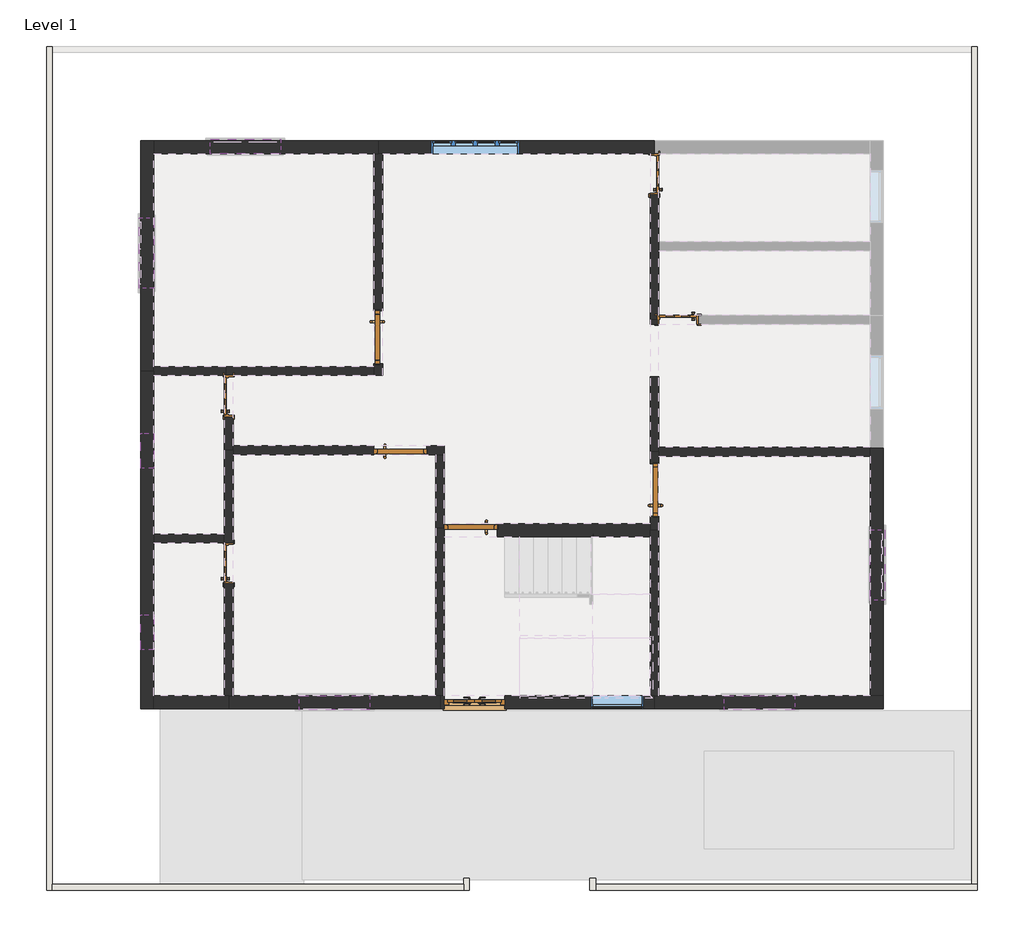
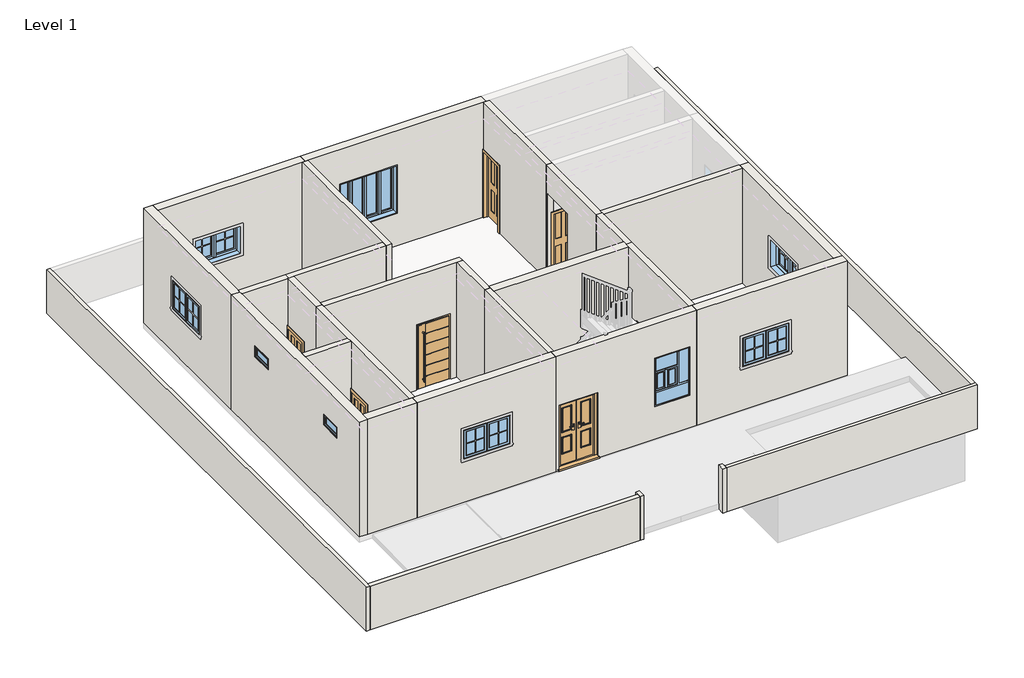
# One storey, part 1 of 2: 30 walls, 9 doors, 9 windows.
"""IFC4 building model written with IfcOpenShell, lengths in millimetres."""

from ifc_helpers import new_model, si_unit, frame, origin, place, context, project, spatial, polyline, outline, extrude, faceted_brep, transform, mapped, element, save
from components import door_3_44036f4b, door_3_3562bf2b, door_a196e7a2, door_f6085f53, door_a03dd1d4, door_7109d6db, m_fixed_2_dd9f9b20, m_window_awning_double_horizontal_4_8afcb0b2, m_window_awning_double_horizontal_4_e2f7b2f6, m_window_casement_double_sash_variable_3_661e274a, m_window_casement_multi_sash_horizontal_5_4f9d37b3

model = new_model("IFC4")

# Units and contexts
model_context = context("Model", 3, world=origin())
ifc_project = project(units=[si_unit("LENGTHUNIT", "METRE", prefix="MILLI")], contexts=[model_context])

# Site, building, storey
site = spatial("IfcSite", under=ifc_project)
building = spatial("IfcBuilding", under=site)
storey = spatial("IfcBuildingStorey", under=building, Name="Level 1", Elevation=0.0)

# Doors
placement = place(None, origin())
door_3_shape = door_3_44036f4b(model_context)
element("IfcDoor", 1, ObjectType="3'", at=placement, inside=storey, context=model_context, shape_type="MappedRepresentation", body=[
    mapped(door_3_shape, transform((-14176.5794909, 1946.4381491, 0.0), x_axis=(0.0, -1.0, 0.0), y_axis=(1.0, 0.0, 0.0), z_axis=(0.0, 0.0, 1.0))),
])
element("IfcDoor", 2, ObjectType="3'", at=placement, inside=storey, context=model_context, shape_type="MappedRepresentation", body=[
    mapped(door_3_shape, transform((-13795.5794909, -9.3618509, 0.0), x_axis=(1.0, 0.0, 0.0), y_axis=(0.0, 1.0, 0.0), z_axis=(0.0, 0.0, 1.0))),
])
element("IfcDoor", 3, ObjectType="3'", at=placement, inside=storey, context=model_context, shape_type="MappedRepresentation", body=[
    mapped(door_3_shape, transform((-9401.3794909, -695.1618509, 0.0), x_axis=(0.0, 1.0, 0.0), y_axis=(-1.0, 0.0, 0.0), z_axis=(0.0, 0.0, 1.0))),
])
door_3_2_shape = door_3_3562bf2b(model_context)
element("IfcDoor", 4, ObjectType="3'", at=placement, inside=storey, context=model_context, shape_type="MappedRepresentation", body=[
    mapped(door_3_2_shape, transform((-12576.3794909, -1393.6618509, 0.0), x_axis=(-1.0, 0.0, 0.0), y_axis=(0.0, -1.0, 0.0), z_axis=(0.0, 0.0, 1.0))),
])
door_shape = door_a196e7a2(model_context)
door_2_shape = door_f6085f53(model_context)
element("IfcDoor", 5, ObjectType="ExtDbl (8) : 3'5\"", at=placement, inside=storey, context=model_context, shape_type="MappedRepresentation", body=[
    mapped(door_shape, transform((-12512.8794909, -4365.4618509, 0.0), x_axis=(-1.0, 0.0, 0.0), y_axis=(0.0, -1.0, 0.0), z_axis=(0.0, 0.0, 1.0))),
    mapped(door_2_shape, transform((-12512.8794909, -4365.4618509, 0.0), x_axis=(-1.0, 0.0, 0.0), y_axis=(0.0, -1.0, 0.0), z_axis=(0.0, 0.0, 1.0))),
])
door_4_shape = door_a03dd1d4(model_context)
element("IfcDoor", 6, ObjectType="M_Door-Interior-Single-4_Panel-Wood : 2'2\"", at=placement, inside=storey, context=model_context, shape_type="MappedRepresentation", body=[
    mapped(door_4_shape, transform((-16770.5544909, 930.8381491, 0.0), x_axis=(0.0, 1.0, 0.0), y_axis=(-1.0, 0.0, 0.0), z_axis=(0.0, 0.0, 1.0))),
])
element("IfcDoor", 7, ObjectType="M_Door-Interior-Single-4_Panel-Wood : 2'2\"", at=placement, inside=storey, context=model_context, shape_type="MappedRepresentation", body=[
    mapped(door_4_shape, transform((-16770.5544909, -1964.7618509, 0.0), x_axis=(0.0, 1.0, 0.0), y_axis=(-1.0, 0.0, 0.0), z_axis=(0.0, 0.0, 1.0))),
])
door_5_shape = door_7109d6db(model_context)
element("IfcDoor", 8, ObjectType="M_Door-Interior-Single-4_Panel-Wood : 2'2\"", at=placement, inside=storey, context=model_context, shape_type="MappedRepresentation", body=[
    mapped(door_5_shape, transform((-8995.3794909, 2254.4131491, 0.0), x_axis=(-1.0, 0.0, 0.0), y_axis=(0.0, -1.0, 0.0), z_axis=(0.0, 0.0, 1.0))),
])
element("IfcDoor", 9, ObjectType="M_Door-Interior-Single-4_Panel-Wood : 2'2\"", at=placement, inside=storey, context=model_context, shape_type="MappedRepresentation", body=[
    mapped(door_5_shape, transform((-9398.2044909, 4766.2381491, 0.0), x_axis=(0.0, 1.0, 0.0), y_axis=(-1.0, 0.0, 0.0), z_axis=(0.0, 0.0, 1.0))),
])

# Walls
element("IfcWall", 10, ObjectType="Generic - 4\"", at=placement, inside=storey, context=model_context, shape_type="Brep", body=[
    faceted_brep([(-19916.9794909, 6975.6381491, -152.4), (-19916.9794909, -7615.8678797, -152.4), (-19916.9794909, -7615.8678797, 1066.8), (-19916.9794909, 6975.6381491, 1066.8), (-19815.3794909, 6975.6381491, -152.4), (-19815.3794909, 6975.6381491, 1066.8), (-19815.3794909, 6874.0381491, 1066.8), (-19815.3794909, -7514.2678797, 1066.8), (-19815.3794909, -7615.8678797, 1066.8), (-19815.3794909, -7615.8678797, -152.4), (-19815.3794909, -7514.2678797, -152.4), (-19815.3794909, 6874.0381491, -152.4)], [[[0, 1, 2, 3]], [[4, 5, 6, 7, 8, 9, 10, 11]], [[1, 0, 4, 11, 10, 9]], [[3, 2, 8, 7, 6, 5]], [[2, 1, 9, 8]], [[0, 3, 5, 4]]]),
])
element("IfcWall", 11, ObjectType="Generic - 4\"", at=placement, inside=storey, context=model_context, shape_type="SweptSolid", body=[
    extrude(outline(polyline([(-12703.3794909, -7615.8678797), (-19815.3794909, -7615.8678797), (-19815.3794909, -7514.2678797), (-12703.3794909, -7514.2678797), (-12703.3794909, -7615.8678797)])), frame((0.0, 0.0, -152.4), z_axis=(0.0, 0.0, 1.0), x_axis=(1.0, 0.0, 0.0)), (0.0, 0.0, 1.0), 1219.2),
])
element("IfcWall", 12, ObjectType="Generic - 4\"", at=placement, inside=storey, context=model_context, shape_type="Brep", body=[
    faceted_brep([(-12601.7794909, -7615.8678797, -152.4), (-12601.7794909, -7412.6678797, -152.4), (-12601.7794909, -7412.6678797, 1066.8), (-12601.7794909, -7615.8678797, 1066.8), (-12703.3794909, -7615.8678797, -152.4), (-12703.3794909, -7615.8678797, 1066.8), (-12703.3794909, -7514.2678797, 1066.8), (-12703.3794909, -7412.6678797, 1066.8), (-12703.3794909, -7412.6678797, -152.4), (-12703.3794909, -7514.2678797, -152.4)], [[[0, 1, 2, 3]], [[4, 5, 6, 7, 8, 9]], [[1, 0, 4, 9, 8]], [[2, 1, 8, 7]], [[3, 2, 7, 6, 5]], [[0, 3, 5, 4]]]),
])
element("IfcWall", 13, ObjectType="Generic - 4\"", at=placement, inside=storey, context=model_context, shape_type="Brep", body=[
    faceted_brep([(-10518.9794909, -7412.6678797, -152.4), (-10518.9794909, -7615.8678797, -152.4), (-10518.9794909, -7615.8678797, 1066.8), (-10518.9794909, -7412.6678797, 1066.8), (-10417.3794909, -7412.6678797, -152.4), (-10417.3794909, -7412.6678797, 1066.8), (-10417.3794909, -7514.2678797, 1066.8), (-10417.3794909, -7615.8678797, 1066.8), (-10417.3794909, -7615.8678797, -152.4), (-10417.3794909, -7514.2678797, -152.4)], [[[0, 1, 2, 3]], [[4, 5, 6, 7, 8, 9]], [[1, 0, 4, 9, 8]], [[3, 2, 7, 6, 5]], [[0, 3, 5, 4]], [[2, 1, 8, 7]]]),
])
element("IfcWall", 14, ObjectType="Generic - 4\"", at=placement, inside=storey, context=model_context, shape_type="Brep", body=[
    faceted_brep([(-10417.3794909, -7615.8678797, -152.4), (-3813.3794909, -7615.8678797, -152.4), (-3813.3794909, -7615.8678797, 1066.8), (-10417.3794909, -7615.8678797, 1066.8), (-10417.3794909, -7514.2678797, -152.4), (-10417.3794909, -7514.2678797, 1066.8), (-3914.9794909, -7514.2678797, 1066.8), (-3813.3794909, -7514.2678797, 1066.8), (-3813.3794909, -7514.2678797, -152.4), (-3914.9794909, -7514.2678797, -152.4)], [[[0, 1, 2, 3]], [[4, 5, 6, 7, 8, 9]], [[1, 0, 4, 9, 8]], [[3, 2, 7, 6, 5]], [[0, 3, 5, 4]], [[2, 1, 8, 7]]]),
])
element("IfcWall", 15, ObjectType="Generic - 4\"", at=placement, inside=storey, context=model_context, shape_type="Brep", body=[
    faceted_brep([(-3813.3794909, -7514.2678797, -152.4), (-3813.3794909, 6975.6381491, -152.4), (-3813.3794909, 6975.6381491, 1066.8), (-3813.3794909, -7514.2678797, 1066.8), (-3914.9794909, -7514.2678797, -152.4), (-3914.9794909, -7514.2678797, 1066.8), (-3914.9794909, 6874.0381491, 1066.8), (-3914.9794909, 6975.6381491, 1066.8), (-3914.9794909, 6975.6381491, -152.4), (-3914.9794909, 6874.0381491, -152.4)], [[[0, 1, 2, 3]], [[4, 5, 6, 7, 8, 9]], [[1, 0, 4, 9, 8]], [[3, 2, 7, 6, 5]], [[0, 3, 5, 4]], [[2, 1, 8, 7]]]),
])
element("IfcWall", 16, ObjectType="Generic - 6\"", at=placement, inside=storey, context=model_context, shape_type="Brep", body=[
    faceted_brep([(-14252.7794909, 1286.0381491, 3200.4), (-14252.7794909, 1438.4381491, 3200.4), (-14252.7794909, 5121.4381491, 3200.4), (-14252.7794909, 5121.4381491, 0.0), (-14252.7794909, 2403.6381491, 0.0), (-14252.7794909, 2403.6381491, 1828.8), (-14252.7794909, 1489.2381491, 1828.8), (-14252.7794909, 1489.2381491, 0.0), (-14252.7794909, 1438.4381491, 0.0), (-14252.7794909, 1286.0381491, 0.0), (-14100.3794909, 5121.4381491, 3200.4), (-14100.3794909, 1286.0381491, 3200.4), (-14100.3794909, 1286.0381491, 0.0), (-14100.3794909, 1489.2381491, 0.0), (-14100.3794909, 1489.2381491, 1828.8), (-14100.3794909, 2403.6381491, 1828.8), (-14100.3794909, 2403.6381491, 0.0), (-14100.3794909, 5121.4381491, 0.0), (-14176.5794909, 5121.4381491, 0.0), (-14155.7794909, 2403.6381491, 0.0), (-14155.7794909, 2418.6381491, 0.0), (-14232.7794909, 2418.6381491, 0.0), (-14232.7794909, 2403.6381491, 0.0), (-14232.7794909, 1489.2381491, 0.0), (-14232.7794909, 1474.2381491, 0.0), (-14155.7794909, 1474.2381491, 0.0), (-14155.7794909, 1489.2381491, 0.0), (-14176.5794909, 5121.4381491, 3200.4), (-14232.7794909, 2403.6381491, 1828.8), (-14232.7794909, 1489.2381491, 1828.8), (-14155.7794909, 1489.2381491, 1828.8), (-14155.7794909, 2403.6381491, 1828.8), (-14232.7794909, 2418.6381491, 1843.8), (-14155.7794909, 2418.6381491, 1843.8), (-14155.7794909, 1474.2381491, 1843.8), (-14232.7794909, 1474.2381491, 1843.8)], [[[0, 1, 2, 3, 4, 5, 6, 7, 8, 9]], [[10, 11, 12, 13, 14, 15, 16, 17]], [[3, 18, 17, 16, 19, 20, 21, 22, 4]], [[12, 9, 8, 7, 23, 24, 25, 26, 13]], [[2, 1, 0, 11, 10, 27]], [[3, 2, 27, 10, 17, 18]], [[0, 9, 12, 11]], [[5, 28, 29, 6]], [[14, 30, 31, 15]], [[6, 29, 23, 7]], [[30, 14, 13, 26]], [[28, 5, 4, 22]], [[15, 31, 19, 16]], [[32, 33, 34, 35]], [[35, 34, 25, 24]], [[31, 30, 26, 25, 34, 33, 20, 19]], [[33, 32, 21, 20]], [[29, 28, 22, 21, 32, 35, 24, 23]]]),
])
element("IfcWall", 17, ObjectType="Generic - 6\"", at=placement, inside=storey, context=model_context, shape_type="Brep", body=[
    faceted_brep([(-14252.7794909, 1438.4381491, 0.0), (-16818.1794909, 1438.4381491, 0.0), (-16818.1794909, 1438.4381491, 3200.4), (-14252.7794909, 1438.4381491, 3200.4), (-14252.7794909, 1286.0381491, 0.0), (-14252.7794909, 1286.0381491, 3200.4), (-16691.1794909, 1286.0381491, 3200.4), (-16818.1794909, 1286.0381491, 3200.4), (-16818.1794909, 1286.0381491, 0.0)], [[[0, 1, 2, 3]], [[4, 5, 6, 7, 8]], [[1, 0, 4, 8]], [[2, 1, 8, 7]], [[3, 2, 7, 6, 5]], [[0, 3, 5, 4]]]),
])
element("IfcWall", 18, ObjectType="Generic - 6\"", at=placement, inside=storey, context=model_context, shape_type="Brep", body=[
    faceted_brep([(-16691.1794909, -9.3618509, 0.0), (-16691.1794909, -9.3618509, 3200.4), (-16691.1794909, -85.5618509, 3200.4), (-16691.1794909, -4251.1618509, 3200.4), (-16691.1794909, -4251.1618509, 0.0), (-16691.1794909, -2319.9618509, 0.0), (-16691.1794909, -2319.9618509, 1853.8), (-16691.1794909, -1609.5618509, 1853.8), (-16691.1794909, -1609.5618509, 0.0), (-16691.1794909, -85.5618509, 0.0), (-16843.5794909, -9.3618509, 3200.4), (-16843.5794909, -9.3618509, 0.0), (-16843.5794909, -1457.1618509, 0.0), (-16843.5794909, -1609.5618509, 0.0), (-16843.5794909, -1609.5618509, 1853.8), (-16843.5794909, -2319.9618509, 1853.8), (-16843.5794909, -2319.9618509, 0.0), (-16843.5794909, -4251.1618509, 0.0), (-16843.5794909, -4251.1618509, 3200.4), (-16843.5794909, -1609.5618509, 3200.4), (-16843.5794909, -1457.1618509, 3200.4), (-16767.3794909, -4251.1618509, 0.0), (-16767.3794909, -4251.1618509, 3200.4)], [[[0, 1, 2, 3, 4, 5, 6, 7, 8, 9]], [[10, 11, 12, 13, 14, 15, 16, 17, 18, 19, 20]], [[4, 21, 17, 16, 5]], [[11, 0, 9, 8, 13, 12]], [[1, 0, 11, 10]], [[3, 2, 1, 10, 20, 19, 18, 22]], [[4, 3, 22, 18, 17, 21]], [[7, 14, 13, 8]], [[14, 7, 6, 15]], [[15, 6, 5, 16]]]),
])
element("IfcWall", 19, ObjectType="Generic - 6\"", at=placement, inside=storey, context=model_context, shape_type="Brep", body=[
    faceted_brep([(-18062.7794909, -1609.5618509, 0.0), (-16843.5794909, -1609.5618509, 0.0), (-16843.5794909, -1609.5618509, 1853.8), (-16843.5794909, -1609.5618509, 3200.4), (-18062.7794909, -1609.5618509, 3200.4), (-18062.7794909, -1457.1618509, 0.0), (-18062.7794909, -1457.1618509, 3200.4), (-16843.5794909, -1457.1618509, 3200.4), (-16843.5794909, -1457.1618509, 0.0)], [[[0, 1, 2, 3, 4]], [[5, 6, 7, 8]], [[1, 0, 5, 8]], [[4, 3, 7, 6]], [[0, 4, 6, 5]], [[3, 2, 1, 8, 7]]]),
])
element("IfcWall", 20, ObjectType="Generic - 6\"", at=placement, inside=storey, context=model_context, shape_type="Brep", body=[
    faceted_brep([(-13033.5794909, -85.5618509, 3200.4), (-13185.9794909, -85.5618509, 3200.4), (-16691.1794909, -85.5618509, 3200.4), (-16691.1794909, -85.5618509, 0.0), (-14252.7794909, -85.5618509, 0.0), (-14252.7794909, -85.5618509, 1828.8), (-13338.3794909, -85.5618509, 1828.8), (-13338.3794909, -85.5618509, 0.0), (-13185.9794909, -85.5618509, 0.0), (-13033.5794909, -85.5618509, 0.0), (-16691.1794909, 66.8381491, 3200.4), (-13033.5794909, 66.8381491, 3200.4), (-13033.5794909, 66.8381491, 0.0), (-13338.3794909, 66.8381491, 0.0), (-13338.3794909, 66.8381491, 1828.8), (-14252.7794909, 66.8381491, 1828.8), (-14252.7794909, 66.8381491, 0.0), (-16691.1794909, 66.8381491, 0.0), (-13338.3794909, -65.5618509, 0.0), (-13323.3794909, -65.5618509, 0.0), (-13323.3794909, 11.4381491, 0.0), (-13338.3794909, 11.4381491, 0.0), (-16691.1794909, -9.3618509, 0.0), (-14252.7794909, 11.4381491, 0.0), (-14267.7794909, 11.4381491, 0.0), (-14267.7794909, -65.5618509, 0.0), (-14252.7794909, -65.5618509, 0.0), (-16691.1794909, -9.3618509, 3200.4), (-14252.7794909, -65.5618509, 1828.8), (-13338.3794909, -65.5618509, 1828.8), (-13338.3794909, 11.4381491, 1828.8), (-14252.7794909, 11.4381491, 1828.8), (-14267.7794909, -65.5618509, 1843.8), (-14267.7794909, 11.4381491, 1843.8), (-13323.3794909, 11.4381491, 1843.8), (-13323.3794909, -65.5618509, 1843.8)], [[[0, 1, 2, 3, 4, 5, 6, 7, 8, 9]], [[10, 11, 12, 13, 14, 15, 16, 17]], [[12, 9, 8, 7, 18, 19, 20, 21, 13]], [[3, 22, 17, 16, 23, 24, 25, 26, 4]], [[2, 1, 0, 11, 10, 27]], [[3, 2, 27, 10, 17, 22]], [[0, 9, 12, 11]], [[5, 28, 29, 6]], [[14, 30, 31, 15]], [[6, 29, 18, 7]], [[30, 14, 13, 21]], [[28, 5, 4, 26]], [[15, 31, 23, 16]], [[32, 33, 34, 35]], [[35, 34, 20, 19]], [[31, 30, 21, 20, 34, 33, 24, 23]], [[33, 32, 25, 24]], [[29, 28, 26, 25, 32, 35, 19, 18]]]),
])
element("IfcWall", 21, ObjectType="Generic - 6\"", at=placement, inside=storey, context=model_context, shape_type="Brep", body=[
    faceted_brep([(-13185.9794909, -85.5618509, 0.0), (-13185.9794909, -1355.5618509, 0.0), (-13185.9794909, -1355.5618509, 3200.4), (-13185.9794909, -85.5618509, 3200.4), (-13033.5794909, -85.5618509, 3200.4), (-13033.5794909, -1355.5618509, 3200.4), (-13033.5794909, -1355.5618509, 1843.8), (-13033.5794909, -1299.3618508, 1843.8), (-13033.5794909, -1299.3618508, 1828.8), (-13033.5794909, -1299.3618508, 0.0), (-13033.5794909, -1279.3618508, 0.0), (-13033.5794909, -85.5618509, 0.0), (-13048.5794909, -1299.3618508, 0.0), (-13048.5794909, -1355.5618509, 0.0), (-13048.5794909, -1355.5618509, 1843.8), (-13048.5794909, -1299.3618508, 1843.8)], [[[0, 1, 2, 3]], [[4, 5, 6, 7, 8, 9, 10, 11]], [[1, 0, 11, 10, 9, 12, 13]], [[2, 1, 13, 14, 6, 5]], [[3, 2, 5, 4]], [[0, 3, 4, 11]], [[14, 15, 7, 6]], [[12, 15, 14, 13]], [[15, 12, 9, 8, 7]]]),
])
element("IfcWall", 22, ObjectType="Generic - 6\"", at=placement, inside=storey, context=model_context, shape_type="Brep", body=[
    faceted_brep([(-9325.1794909, -4251.1618509, 0.0), (-9325.1794909, -1393.6618509, 0.0), (-9325.1794909, -1393.6618509, 3200.4), (-9325.1794909, -4251.1618509, 3200.4), (-9477.5794909, -4251.1618509, 0.0), (-9477.5794909, -4251.1618509, 3200.4), (-9477.5794909, -1507.9618509, 3200.4), (-9477.5794909, -1393.6618509, 3200.4), (-9477.5794909, -1393.6618509, 0.0), (-9477.5794909, -1507.9618509, 0.0), (-9401.3794909, -4251.1618509, 0.0), (-9401.3794909, -4251.1618509, 3200.4)], [[[0, 1, 2, 3]], [[4, 5, 6, 7, 8, 9]], [[1, 0, 10, 4, 9, 8]], [[2, 1, 8, 7]], [[3, 2, 7, 6, 5, 11]], [[0, 3, 11, 5, 4, 10]]]),
])
element("IfcWall", 23, ObjectType="Generic - 6\"", at=placement, inside=storey, context=model_context, shape_type="Brep", body=[
    faceted_brep([(-5667.5794909, 41.4381491, 0.0), (-9325.1794909, 41.4381491, 0.0), (-9325.1794909, 41.4381491, 3200.4), (-5667.5794909, 41.4381491, 3200.4), (-5667.5794909, -110.9618509, 0.0), (-5667.5794909, -110.9618509, 3200.4), (-9325.1794909, -110.9618509, 3200.4), (-9325.1794909, -110.9618509, 0.0), (-5667.5794909, 28.7381491, 0.0), (-9325.1794909, -34.7618509, 0.0), (-9325.1794909, -34.7618509, 3200.4), (-5667.5794909, 28.7381491, 3200.4)], [[[0, 1, 2, 3]], [[4, 5, 6, 7]], [[1, 0, 8, 4, 7, 9]], [[3, 2, 10, 6, 5, 11]], [[0, 3, 11, 5, 4, 8]], [[2, 1, 9, 7, 6, 10]]]),
])
element("IfcWall", 24, ObjectType="Generic - 6\"", at=placement, inside=storey, context=model_context, shape_type="Brep", body=[
    faceted_brep([(-16691.1794909, 1286.0381491, 3200.4), (-16691.1794909, 66.8381491, 3200.4), (-16691.1794909, -9.3618509, 3200.4), (-16691.1794909, -9.3618509, 0.0), (-16691.1794909, 66.8381491, 0.0), (-16691.1794909, 575.6381491, 0.0), (-16691.1794909, 575.6381491, 1853.8), (-16691.1794909, 1286.0381491, 1853.8), (-16843.5794909, -9.3618509, 3200.4), (-16843.5794909, 1286.0381491, 3200.4), (-16843.5794909, 1286.0381491, 1853.8), (-16843.5794909, 575.6381491, 1853.8), (-16843.5794909, 575.6381491, 0.0), (-16843.5794909, -9.3618509, 0.0), (-16818.1794909, 1286.0381491, 3200.4)], [[[0, 1, 2, 3, 4, 5, 6, 7]], [[8, 9, 10, 11, 12, 13]], [[3, 13, 12, 5, 4]], [[2, 1, 0, 14, 9, 8]], [[3, 2, 8, 13]], [[9, 14, 0, 7, 10]], [[6, 11, 10, 7]], [[11, 6, 5, 12]]]),
])
element("IfcWall", 25, ObjectType="Generic - 6\"", at=placement, inside=storey, context=model_context, shape_type="Brep", body=[
    faceted_brep([(-9325.1794909, 2251.2381491, 3200.4), (-9325.1794909, 2175.0381491, 3200.4), (-9325.1794909, 41.4381491, 3200.4), (-9325.1794909, -34.7618509, 3200.4), (-9325.1794909, -34.7618509, 0.0), (-9325.1794909, 41.4381491, 0.0), (-9325.1794909, 1260.4626795, 0.0), (-9325.1794909, 1260.4626795, 2438.4), (-9325.1794909, 2175.0381491, 2438.4), (-9325.1794909, 2175.0381491, 1853.8), (-9325.1794909, 2251.2381491, 1853.8), (-9477.5794909, 2251.2381491, 3200.4), (-9477.5794909, 2251.2381491, 0.0), (-9477.5794909, 2175.0381491, 0.0), (-9477.5794909, 2175.0381491, 2438.4), (-9477.5794909, 1260.4626795, 2438.4), (-9477.5794909, 1260.4626795, 0.0), (-9477.5794909, -34.7618509, 0.0), (-9477.5794909, -34.7618509, 3200.4), (-9350.5794909, 2251.2381491, 0.0), (-9350.5794909, 2175.0381491, 0.0), (-9350.5794909, 2251.2381491, 1853.8), (-9350.5794909, 2175.0381491, 1853.8)], [[[0, 1, 2, 3, 4, 5, 6, 7, 8, 9, 10]], [[11, 12, 13, 14, 15, 16, 17, 18]], [[13, 12, 19, 20]], [[4, 17, 16, 6, 5]], [[12, 11, 0, 10, 21, 19]], [[3, 2, 1, 0, 11, 18]], [[4, 3, 18, 17]], [[7, 15, 14, 8]], [[15, 7, 6, 16]], [[8, 14, 13, 20, 22, 9]], [[21, 22, 20, 19]], [[22, 21, 10, 9]]]),
])
element("IfcWall", 26, ObjectType="Generic - 6\"", at=placement, inside=storey, context=model_context, shape_type="Brep", body=[
    faceted_brep([(-16818.1794909, 1438.4381491, 0.0), (-18062.7794909, 1438.4381491, 0.0), (-18062.7794909, 1438.4381491, 3200.4), (-16818.1794909, 1438.4381491, 3200.4), (-16818.1794909, 1286.0381491, 0.0), (-16818.1794909, 1286.0381491, 3200.4), (-18062.7794909, 1286.0381491, 3200.4), (-18062.7794909, 1286.0381491, 0.0), (-18062.7794909, 1362.2381491, 0.0), (-18062.7794909, 1362.2381491, 3200.4)], [[[0, 1, 2, 3]], [[4, 5, 6, 7]], [[1, 0, 4, 7, 8]], [[3, 2, 9, 6, 5]], [[0, 3, 5, 4]], [[2, 1, 8, 7, 6, 9]]]),
])
element("IfcWall", 27, ObjectType="Generic - 6\"", at=placement, inside=storey, context=model_context, shape_type="Brep", body=[
    faceted_brep([(-13185.9794909, -1355.5618509, 0.0), (-13185.9794909, -4251.1618509, 0.0), (-13185.9794909, -4251.1618509, 3200.4), (-13185.9794909, -1355.5618509, 3200.4), (-13033.5794909, -1355.5618509, 3200.4), (-13033.5794909, -1507.9618509, 3200.4), (-13033.5794909, -4251.1618509, 3200.4), (-13033.5794909, -4251.1618509, 1828.8), (-13033.5794909, -4251.1618509, 0.0), (-13033.5794909, -1507.9618509, 0.0), (-13033.5794909, -1376.3618508, 0.0), (-13033.5794909, -1376.3618508, 1828.8), (-13033.5794909, -1376.3618508, 1843.8), (-13033.5794909, -1355.5618509, 1843.8), (-13048.5794909, -1355.5618509, 0.0), (-13048.5794909, -1376.3618508, 0.0), (-13109.7794909, -4251.1618509, 0.0), (-13109.7794909, -4251.1618509, 3200.4), (-13048.5794909, -1355.5618509, 1843.8), (-13048.5794909, -1376.3618508, 1843.8)], [[[0, 1, 2, 3]], [[4, 5, 6, 7, 8, 9, 10, 11, 12, 13]], [[1, 0, 14, 15, 10, 9, 8, 16]], [[3, 2, 17, 6, 5, 4]], [[0, 3, 4, 13, 18, 14]], [[2, 1, 16, 8, 7, 6, 17]], [[12, 19, 18, 13]], [[19, 15, 14, 18]], [[15, 19, 12, 11, 10]]]),
])
element("IfcWall", 28, ObjectType="Generic - 6\"", at=placement, inside=storey, context=model_context, shape_type="Brep", body=[
    faceted_brep([(-9325.1794909, -34.7618509, 0.0), (-9325.1794909, -34.7618509, 3200.4), (-9325.1794909, -110.9618509, 3200.4), (-9325.1794909, -1393.6618509, 3200.4), (-9325.1794909, -1393.6618509, 0.0), (-9325.1794909, -1152.3618509, 0.0), (-9325.1794909, -1152.3618509, 1828.8), (-9325.1794909, -237.9618509, 1828.8), (-9325.1794909, -237.9618509, 0.0), (-9325.1794909, -110.9618509, 0.0), (-9477.5794909, -34.7618509, 3200.4), (-9477.5794909, -34.7618509, 0.0), (-9477.5794909, -237.9618509, 0.0), (-9477.5794909, -237.9618509, 1828.8), (-9477.5794909, -1152.3618509, 1828.8), (-9477.5794909, -1152.3618509, 0.0), (-9477.5794909, -1279.3618509, 0.0), (-9477.5794909, -1393.6618509, 0.0), (-9477.5794909, -1393.6618509, 3200.4), (-9477.5794909, -1279.3618509, 3200.4), (-9345.1794909, -237.9618509, 0.0), (-9345.1794909, -222.9618509, 0.0), (-9422.1794909, -222.9618509, 0.0), (-9422.1794909, -237.9618509, 0.0), (-9422.1794909, -1152.3618509, 0.0), (-9422.1794909, -1167.3618509, 0.0), (-9345.1794909, -1167.3618509, 0.0), (-9345.1794909, -1152.3618509, 0.0), (-9345.1794909, -1152.3618509, 1828.8), (-9345.1794909, -237.9618509, 1828.8), (-9422.1794909, -237.9618509, 1828.8), (-9422.1794909, -1152.3618509, 1828.8), (-9345.1794909, -1167.3618509, 1843.8), (-9422.1794909, -1167.3618509, 1843.8), (-9422.1794909, -222.9618509, 1843.8), (-9345.1794909, -222.9618509, 1843.8)], [[[0, 1, 2, 3, 4, 5, 6, 7, 8, 9]], [[10, 11, 12, 13, 14, 15, 16, 17, 18, 19]], [[11, 0, 9, 8, 20, 21, 22, 23, 12]], [[4, 17, 16, 15, 24, 25, 26, 27, 5]], [[1, 0, 11, 10]], [[3, 2, 1, 10, 19, 18]], [[4, 3, 18, 17]], [[6, 28, 29, 7]], [[13, 30, 31, 14]], [[30, 13, 12, 23]], [[7, 29, 20, 8]], [[14, 31, 24, 15]], [[28, 6, 5, 27]], [[32, 33, 34, 35]], [[35, 34, 22, 21]], [[31, 30, 23, 22, 34, 33, 25, 24]], [[33, 32, 26, 25]], [[29, 28, 27, 26, 32, 35, 21, 20]]]),
])
element("IfcWall", 29, ObjectType="Generic - 6\"", at=placement, inside=storey, context=model_context, shape_type="Brep", body=[
    faceted_brep([(-9325.1794909, 5121.4381491, 3200.4), (-9325.1794909, 3597.4381491, 3200.4), (-9325.1794909, 3445.0381491, 3200.4), (-9325.1794909, 2327.4381491, 3200.4), (-9325.1794909, 2251.2381491, 3200.4), (-9325.1794909, 2251.2381491, 1853.8), (-9325.1794909, 2327.4381491, 1853.8), (-9325.1794909, 2327.4381491, 0.0), (-9325.1794909, 3445.0381491, 0.0), (-9325.1794909, 3597.4381491, 0.0), (-9325.1794909, 4411.0381491, 0.0), (-9325.1794909, 4411.0381491, 1853.8), (-9325.1794909, 5121.4381491, 1853.8), (-9477.5794909, 2251.2381491, 3200.4), (-9477.5794909, 5121.4381491, 3200.4), (-9477.5794909, 5121.4381491, 1853.8), (-9477.5794909, 4411.0381491, 1853.8), (-9477.5794909, 4411.0381491, 0.0), (-9477.5794909, 2251.2381491, 0.0), (-9350.5794909, 2327.4381491, 0.0), (-9350.5794909, 2251.2381491, 0.0), (-9401.3794909, 5121.4381491, 3200.4), (-9350.5794909, 2251.2381491, 1853.8), (-9350.5794909, 2327.4381491, 1853.8)], [[[0, 1, 2, 3, 4, 5, 6, 7, 8, 9, 10, 11, 12]], [[13, 14, 15, 16, 17, 18]], [[18, 17, 10, 9, 8, 7, 19, 20]], [[4, 3, 2, 1, 0, 21, 14, 13]], [[13, 18, 20, 22, 5, 4]], [[14, 21, 0, 12, 15]], [[11, 16, 15, 12]], [[16, 11, 10, 17]], [[23, 19, 7, 6]], [[19, 23, 22, 20]], [[23, 6, 5, 22]]]),
])
element("IfcWall", 30, ObjectType="Generic - 9\"", at=placement, inside=storey, context=model_context, shape_type="Brep", body=[
    faceted_brep([(-18291.3794909, 5350.0381491, 0.0), (-18291.3794909, 1362.2381491, 0.0), (-18291.3794909, 1362.2381491, 3200.4), (-18291.3794909, 5350.0381491, 3200.4), (-18291.3794909, 4011.7756491, 2019.2), (-18291.3794909, 2792.5756491, 2019.2), (-18291.3794909, 2792.5756491, 1219.2), (-18291.3794909, 4011.7756491, 1219.2), (-18062.7794909, 5350.0381491, 0.0), (-18062.7794909, 5350.0381491, 3200.4), (-18062.7794909, 5121.4381491, 3200.4), (-18062.7794909, 1438.4381491, 3200.4), (-18062.7794909, 1362.2381491, 3200.4), (-18062.7794909, 1362.2381491, 0.0), (-18062.7794909, 1438.4381491, 0.0), (-18062.7794909, 5121.4381491, 0.0), (-18062.7794909, 4011.7756491, 2019.2), (-18062.7794909, 4011.7756491, 1219.2), (-18062.7794909, 2792.5756491, 1219.2), (-18062.7794909, 2792.5756491, 2019.2)], [[[0, 1, 2, 3], [4, 5, 6, 7]], [[8, 9, 10, 11, 12, 13, 14, 15], [16, 17, 18, 19]], [[1, 0, 8, 15, 14, 13]], [[2, 1, 13, 12]], [[3, 2, 12, 11, 10, 9]], [[0, 3, 9, 8]], [[17, 16, 4, 7]], [[18, 17, 7, 6]], [[19, 18, 6, 5]], [[16, 19, 5, 4]]]),
])
element("IfcWall", 31, ObjectType="Generic - 9\"", at=placement, inside=storey, context=model_context, shape_type="Brep", body=[
    faceted_brep([(-18062.7794909, -4479.7618509, 0.0), (-16767.3794909, -4479.7618509, 0.0), (-16767.3794909, -4479.7618509, 3200.4), (-18062.7794909, -4479.7618509, 3200.4), (-18062.7794909, -4251.1618509, 0.0), (-18062.7794909, -4251.1618509, 3200.4), (-16843.5794909, -4251.1618509, 3200.4), (-16767.3794909, -4251.1618509, 3200.4), (-16767.3794909, -4251.1618509, 0.0), (-16843.5794909, -4251.1618509, 0.0)], [[[0, 1, 2, 3]], [[4, 5, 6, 7, 8, 9]], [[1, 0, 4, 9, 8]], [[2, 1, 8, 7]], [[3, 2, 7, 6, 5]], [[0, 3, 5, 4]]]),
])
element("IfcWall", 32, ObjectType="Generic - 9\"", at=placement, inside=storey, context=model_context, shape_type="Brep", body=[
    faceted_brep([(-5438.9794909, -4251.1618509, 0.0), (-5438.9794909, 28.7381491, 0.0), (-5438.9794909, 28.7381491, 3200.4), (-5438.9794909, -4251.1618509, 3200.4), (-5438.9794909, -2600.1618509, 2019.2), (-5438.9794909, -1380.9618509, 2019.2), (-5438.9794909, -1380.9618509, 1219.2), (-5438.9794909, -2600.1618509, 1219.2), (-5667.5794909, -4251.1618509, 0.0), (-5667.5794909, -4251.1618509, 3200.4), (-5667.5794909, -110.9618509, 3200.4), (-5667.5794909, 28.7381491, 3200.4), (-5667.5794909, 28.7381491, 0.0), (-5667.5794909, -110.9618509, 0.0), (-5667.5794909, -2600.1618509, 2019.2), (-5667.5794909, -2600.1618509, 1219.2), (-5667.5794909, -1380.9618509, 1219.2), (-5667.5794909, -1380.9618509, 2019.2)], [[[0, 1, 2, 3], [4, 5, 6, 7]], [[8, 9, 10, 11, 12, 13], [14, 15, 16, 17]], [[1, 0, 8, 13, 12]], [[2, 1, 12, 11]], [[3, 2, 11, 10, 9]], [[0, 3, 9, 8]], [[15, 14, 4, 7]], [[16, 15, 7, 6]], [[17, 16, 6, 5]], [[14, 17, 5, 4]]]),
])
element("IfcWall", 33, ObjectType="Generic - 9\"", at=placement, inside=storey, context=model_context, shape_type="Brep", body=[
    faceted_brep([(-13033.5794909, -1279.3618509, 3200.4), (-9477.5794909, -1279.3618509, 3200.4), (-9477.5794909, -1279.3618509, 0.0), (-12119.1794909, -1279.3618509, 0.0), (-12119.1794909, -1279.3618509, 1828.8), (-13033.5794909, -1279.3618509, 1828.8), (-9477.5794909, -1507.9618509, 3200.4), (-13033.5794909, -1507.9618509, 3200.4), (-13033.5794909, -1507.9618509, 1828.8), (-12119.1794909, -1507.9618509, 1828.8), (-12119.1794909, -1507.9618509, 0.0), (-9477.5794909, -1507.9618509, 0.0), (-9477.5794909, -1393.6618509, 0.0), (-12119.1794909, -1376.3618508, 0.0), (-12104.1794909, -1376.3618508, 0.0), (-12104.1794909, -1299.3618508, 0.0), (-12119.1794909, -1299.3618508, 0.0), (-13033.5794909, -1355.5618509, 3200.4), (-9477.5794909, -1393.6618509, 3200.4), (-13033.5794909, -1299.3618508, 1828.8), (-13033.5794909, -1299.3618508, 1843.8), (-13033.5794909, -1355.5618509, 1843.8), (-13033.5794909, -1376.3618508, 1843.8), (-13033.5794909, -1376.3618508, 1828.8), (-12119.1794909, -1299.3618508, 1828.8), (-12119.1794909, -1376.3618508, 1828.8), (-12104.1794909, -1299.3618508, 1843.8), (-12104.1794909, -1376.3618508, 1843.8)], [[[0, 1, 2, 3, 4, 5]], [[6, 7, 8, 9, 10, 11]], [[2, 12, 11, 10, 13, 14, 15, 16, 3]], [[1, 0, 17, 7, 6, 18]], [[7, 17, 0, 5, 19, 20, 21, 22, 23, 8]], [[2, 1, 18, 6, 11, 12]], [[4, 24, 19, 5]], [[23, 25, 9, 8]], [[24, 4, 3, 16]], [[9, 25, 13, 10]], [[26, 27, 22, 21, 20]], [[25, 23, 22, 27, 14, 13]], [[27, 26, 15, 14]], [[19, 24, 16, 15, 26, 20]]]),
])
element("IfcWall", 34, ObjectType="Generic - 9\"", at=placement, inside=storey, context=model_context, shape_type="Brep", body=[
    faceted_brep([(-14176.5794909, 5350.0381491, 0.0), (-18062.7794909, 5350.0381491, 0.0), (-18062.7794909, 5350.0381491, 3200.4), (-14176.5794909, 5350.0381491, 3200.4), (-17088.0544909, 5350.0381491, 2019.2), (-17088.0544909, 5350.0381491, 1219.2), (-15868.8544909, 5350.0381491, 1219.2), (-15868.8544909, 5350.0381491, 2019.2), (-14176.5794909, 5121.4381491, 0.0), (-14176.5794909, 5121.4381491, 3200.4), (-14252.7794909, 5121.4381491, 3200.4), (-18062.7794909, 5121.4381491, 3200.4), (-18062.7794909, 5121.4381491, 0.0), (-14252.7794909, 5121.4381491, 0.0), (-17088.0544909, 5121.4381491, 2019.2), (-15868.8544909, 5121.4381491, 2019.2), (-15868.8544909, 5121.4381491, 1219.2), (-17088.0544909, 5121.4381491, 1219.2)], [[[0, 1, 2, 3], [4, 5, 6, 7]], [[8, 9, 10, 11, 12, 13], [14, 15, 16, 17]], [[1, 0, 8, 13, 12]], [[3, 2, 11, 10, 9]], [[0, 3, 9, 8]], [[2, 1, 12, 11]], [[4, 7, 15, 14]], [[7, 6, 16, 15]], [[6, 5, 17, 16]], [[5, 4, 14, 17]]]),
])
element("IfcWall", 35, ObjectType="Generic - 9\"", at=placement, inside=storey, context=model_context, shape_type="Brep", body=[
    faceted_brep([(-9401.3794909, 5350.0381491, 0.0), (-14176.5794909, 5350.0381491, 0.0), (-14176.5794909, 5350.0381491, 3200.4), (-9401.3794909, 5350.0381491, 3200.4), (-11741.3544909, 5350.0381491, 2250.0), (-13265.3544909, 5350.0381491, 2250.0), (-13265.3544909, 5350.0381491, 900.0), (-11741.3544909, 5350.0381491, 900.0), (-9401.3794909, 5121.4381491, 0.0), (-9401.3794909, 5121.4381491, 3200.4), (-9477.5794909, 5121.4381491, 3200.4), (-14100.3794909, 5121.4381491, 3200.4), (-14176.5794909, 5121.4381491, 3200.4), (-14176.5794909, 5121.4381491, 0.0), (-14100.3794909, 5121.4381491, 0.0), (-11741.3544909, 5121.4381491, 2250.0), (-11741.3544909, 5121.4381491, 900.0), (-13265.3544909, 5121.4381491, 900.0), (-13265.3544909, 5121.4381491, 2250.0)], [[[0, 1, 2, 3], [4, 5, 6, 7]], [[8, 9, 10, 11, 12, 13, 14], [15, 16, 17, 18]], [[1, 0, 8, 14, 13]], [[2, 1, 13, 12]], [[3, 2, 12, 11, 10, 9]], [[0, 3, 9, 8]], [[15, 18, 5, 4]], [[18, 17, 6, 5]], [[17, 16, 7, 6]], [[16, 15, 4, 7]]]),
])
element("IfcWall", 36, ObjectType="Generic - 9\"", at=placement, inside=storey, context=model_context, shape_type="Brep", body=[
    faceted_brep([(-18291.3794909, 1362.2381491, 0.0), (-18291.3794909, -4479.7618509, 0.0), (-18291.3794909, -4479.7618509, 3200.4), (-18291.3794909, 1362.2381491, 3200.4), (-18291.3794909, -3462.9681009, 2133.6), (-18291.3794909, -2853.3681009, 2133.6), (-18291.3794909, -2853.3681009, 2438.4), (-18291.3794909, -3462.9681009, 2438.4), (-18291.3794909, -321.3056009, 2133.6), (-18291.3794909, 288.2943991, 2133.6), (-18291.3794909, 288.2943991, 2438.4), (-18291.3794909, -321.3056009, 2438.4), (-18062.7794909, 1362.2381491, 0.0), (-18062.7794909, 1362.2381491, 3200.4), (-18062.7794909, 1286.0381491, 3200.4), (-18062.7794909, -1457.1618509, 3200.4), (-18062.7794909, -1609.5618509, 3200.4), (-18062.7794909, -4251.1618509, 3200.4), (-18062.7794909, -4479.7618509, 3200.4), (-18062.7794909, -4479.7618509, 0.0), (-18062.7794909, -4251.1618509, 0.0), (-18062.7794909, -1609.5618509, 0.0), (-18062.7794909, -1457.1618509, 0.0), (-18062.7794909, 1286.0381491, 0.0), (-18062.7794909, -3462.9681009, 2133.6), (-18062.7794909, -3462.9681009, 2438.4), (-18062.7794909, -2853.3681009, 2438.4), (-18062.7794909, -2853.3681009, 2133.6), (-18062.7794909, -321.3056009, 2133.6), (-18062.7794909, -321.3056009, 2438.4), (-18062.7794909, 288.2943991, 2438.4), (-18062.7794909, 288.2943991, 2133.6)], [[[0, 1, 2, 3], [4, 5, 6, 7], [8, 9, 10, 11]], [[12, 13, 14, 15, 16, 17, 18, 19, 20, 21, 22, 23], [24, 25, 26, 27], [28, 29, 30, 31]], [[1, 0, 12, 23, 22, 21, 20, 19]], [[3, 2, 18, 17, 16, 15, 14, 13]], [[0, 3, 13, 12]], [[2, 1, 19, 18]], [[24, 27, 5, 4]], [[27, 26, 6, 5]], [[26, 25, 7, 6]], [[25, 24, 4, 7]], [[28, 31, 9, 8]], [[31, 30, 10, 9]], [[30, 29, 11, 10]], [[29, 28, 8, 11]]]),
])
element("IfcWall", 37, ObjectType="Generic - 9\"", at=placement, inside=storey, context=model_context, shape_type="Brep", body=[
    faceted_brep([(-16767.3794909, -4479.7618509, 0.0), (-13109.7794909, -4479.7618509, 0.0), (-13109.7794909, -4479.7618509, 3200.4), (-16767.3794909, -4479.7618509, 3200.4), (-15544.2107409, -4479.7618509, 2019.2), (-14325.0107409, -4479.7618509, 2019.2), (-14325.0107409, -4479.7618509, 1219.2), (-15544.2107409, -4479.7618509, 1219.2), (-16767.3794909, -4251.1618509, 0.0), (-16767.3794909, -4251.1618509, 3200.4), (-16691.1794909, -4251.1618509, 3200.4), (-13185.9794909, -4251.1618509, 3200.4), (-13109.7794909, -4251.1618509, 3200.4), (-13109.7794909, -4251.1618509, 0.0), (-13185.9794909, -4251.1618509, 0.0), (-16691.1794909, -4251.1618509, 0.0), (-15544.2107409, -4251.1618509, 2019.2), (-15544.2107409, -4251.1618509, 1219.2), (-14325.0107409, -4251.1618509, 1219.2), (-14325.0107409, -4251.1618509, 2019.2)], [[[0, 1, 2, 3], [4, 5, 6, 7]], [[8, 9, 10, 11, 12, 13, 14, 15], [16, 17, 18, 19]], [[1, 0, 8, 15, 14, 13]], [[2, 1, 13, 12]], [[3, 2, 12, 11, 10, 9]], [[0, 3, 9, 8]], [[16, 19, 5, 4]], [[19, 18, 6, 5]], [[18, 17, 7, 6]], [[17, 16, 4, 7]]]),
])
element("IfcWall", 38, ObjectType="Generic - 9\"", at=placement, inside=storey, context=model_context, shape_type="Brep", body=[
    faceted_brep([(-9401.3794909, -4479.7618509, 0.0), (-5438.9794909, -4479.7618509, 0.0), (-5438.9794909, -4479.7618509, 3200.4), (-9401.3794909, -4479.7618509, 3200.4), (-8196.4669909, -4479.7618509, 2019.2), (-6977.2669909, -4479.7618509, 2019.2), (-6977.2669909, -4479.7618509, 1219.2), (-8196.4669909, -4479.7618509, 1219.2), (-9401.3794909, -4251.1618509, 0.0), (-9401.3794909, -4251.1618509, 3200.4), (-9325.1794909, -4251.1618509, 3200.4), (-5667.5794909, -4251.1618509, 3200.4), (-5438.9794909, -4251.1618509, 3200.4), (-5438.9794909, -4251.1618509, 0.0), (-5667.5794909, -4251.1618509, 0.0), (-9325.1794909, -4251.1618509, 0.0), (-8196.4669909, -4251.1618509, 2019.2), (-8196.4669909, -4251.1618509, 1219.2), (-6977.2669909, -4251.1618509, 1219.2), (-6977.2669909, -4251.1618509, 2019.2)], [[[0, 1, 2, 3], [4, 5, 6, 7]], [[8, 9, 10, 11, 12, 13, 14, 15], [16, 17, 18, 19]], [[1, 0, 8, 15, 14, 13]], [[3, 2, 12, 11, 10, 9]], [[0, 3, 9, 8]], [[2, 1, 13, 12]], [[16, 19, 5, 4]], [[19, 18, 6, 5]], [[18, 17, 7, 6]], [[17, 16, 4, 7]]]),
])
element("IfcWall", 39, ObjectType="Generic - 9\"", at=placement, inside=storey, context=model_context, shape_type="Brep", body=[
    faceted_brep([(-13109.7794909, -4479.7618509, 0.0), (-13033.5794909, -4479.7618509, 0.0), (-13033.5794909, -4479.7618509, 1828.8), (-11992.1794909, -4479.7618509, 1828.8), (-11992.1794909, -4479.7618509, 0.0), (-9401.3794909, -4479.7618509, 0.0), (-9401.3794909, -4479.7618509, 3200.4), (-13109.7794909, -4479.7618509, 3200.4), (-10499.9294909, -4479.7618509, 2250.0), (-9585.5294909, -4479.7618509, 2250.0), (-9585.5294909, -4479.7618509, 900.0), (-10499.9294909, -4479.7618509, 900.0), (-13033.5794909, -4251.1618509, 1828.8), (-13033.5794909, -4251.1618509, 0.0), (-13109.7794909, -4251.1618509, 0.0), (-13109.7794909, -4251.1618509, 3200.4), (-13033.5794909, -4251.1618509, 3200.4), (-9477.5794909, -4251.1618509, 3200.4), (-9401.3794909, -4251.1618509, 3200.4), (-9401.3794909, -4251.1618509, 0.0), (-9477.5794909, -4251.1618509, 0.0), (-11992.1794909, -4251.1618509, 0.0), (-11992.1794909, -4251.1618509, 1828.8), (-10499.9294909, -4251.1618509, 2250.0), (-10499.9294909, -4251.1618509, 900.0), (-9585.5294909, -4251.1618509, 900.0), (-9585.5294909, -4251.1618509, 2250.0)], [[[0, 1, 2, 3, 4, 5, 6, 7], [8, 9, 10, 11]], [[12, 13, 14, 15, 16, 17, 18, 19, 20, 21, 22], [23, 24, 25, 26]], [[14, 13, 1, 0]], [[21, 20, 19, 5, 4]], [[6, 5, 19, 18]], [[7, 6, 18, 17, 16, 15]], [[0, 7, 15, 14]], [[3, 2, 12, 22]], [[2, 1, 13, 12]], [[4, 3, 22, 21]], [[23, 26, 9, 8]], [[26, 25, 10, 9]], [[25, 24, 11, 10]], [[24, 23, 8, 11]]]),
])

# Windows
m_fixed_2_shape = m_fixed_2_dd9f9b20(model_context)
element("IfcWindow", 40, ObjectType="M_Fixed : 2'", at=placement, inside=storey, context=model_context, shape_type="MappedRepresentation", body=[
    mapped(m_fixed_2_shape, transform((-18164.0794909, -3158.1681009, 1218.6), x_axis=(0.0, 1.0, 0.0), y_axis=(-1.0, 0.0, 0.0), z_axis=(0.0, 0.0, 1.0))),
])
element("IfcWindow", 41, ObjectType="M_Fixed : 2'", at=placement, inside=storey, context=model_context, shape_type="MappedRepresentation", body=[
    mapped(m_fixed_2_shape, transform((-18164.0794909, -16.5056009, 1218.6), x_axis=(0.0, 1.0, 0.0), y_axis=(-1.0, 0.0, 0.0), z_axis=(0.0, 0.0, 1.0))),
])
m_window_awning_double_horizontal_4_shape = m_window_awning_double_horizontal_4_8afcb0b2(model_context)
element("IfcWindow", 42, ObjectType="M_Window-Awning-Double-Horizontal : 4'", at=placement, inside=storey, context=model_context, shape_type="MappedRepresentation", body=[
    mapped(m_window_awning_double_horizontal_4_shape, transform((-18177.0794909, 3402.1756491, 319.2), x_axis=(0.0, 1.0, 0.0), y_axis=(-1.0, 0.0, 0.0), z_axis=(0.0, 0.0, 1.0))),
])
element("IfcWindow", 43, ObjectType="M_Window-Awning-Double-Horizontal : 4'", at=placement, inside=storey, context=model_context, shape_type="MappedRepresentation", body=[
    mapped(m_window_awning_double_horizontal_4_shape, transform((-5553.2794909, -1990.5618509, 319.2), x_axis=(0.0, -1.0, 0.0), y_axis=(1.0, 0.0, 0.0), z_axis=(0.0, 0.0, 1.0))),
])
element("IfcWindow", 44, ObjectType="M_Window-Awning-Double-Horizontal : 4'", at=placement, inside=storey, context=model_context, shape_type="MappedRepresentation", body=[
    mapped(m_window_awning_double_horizontal_4_shape, transform((-7586.8669909, -4365.4618509, 319.2), x_axis=(-1.0, 0.0, 0.0), y_axis=(0.0, -1.0, 0.0), z_axis=(0.0, 0.0, 1.0))),
])
element("IfcWindow", 45, ObjectType="M_Window-Awning-Double-Horizontal : 4'", at=placement, inside=storey, context=model_context, shape_type="MappedRepresentation", body=[
    mapped(m_window_awning_double_horizontal_4_shape, transform((-14934.6107409, -4365.4618509, 319.2), x_axis=(-1.0, 0.0, 0.0), y_axis=(0.0, -1.0, 0.0), z_axis=(0.0, 0.0, 1.0))),
])
m_window_awning_double_horizontal_4_2_shape = m_window_awning_double_horizontal_4_e2f7b2f6(model_context)
element("IfcWindow", 46, ObjectType="M_Window-Awning-Double-Horizontal : 4'", at=placement, inside=storey, context=model_context, shape_type="MappedRepresentation", body=[
    mapped(m_window_awning_double_horizontal_4_2_shape, transform((-16478.4544909, 5235.7381491, 319.2), x_axis=(-1.0, 0.0, 0.0), y_axis=(0.0, -1.0, 0.0), z_axis=(0.0, 0.0, 1.0))),
])
m_window_casement_double_sash_variable_3_shape = m_window_casement_double_sash_variable_3_661e274a(model_context)
element("IfcWindow", 47, ObjectType="M_Window-Casement-Double-Sash-Variable : 3'", at=placement, inside=storey, context=model_context, shape_type="MappedRepresentation", body=[
    mapped(m_window_casement_double_sash_variable_3_shape, transform((-10042.7294909, -4365.4618509, 0.0), x_axis=(-1.0, 0.0, 0.0), y_axis=(0.0, -1.0, 0.0), z_axis=(0.0, 0.0, 1.0))),
])
m_window_casement_multi_sash_horizontal_5_shape = m_window_casement_multi_sash_horizontal_5_4f9d37b3(model_context)
element("IfcWindow", 48, ObjectType="M_Window-Casement-Multi-Sash-Horizontal : 5'", at=placement, inside=storey, context=model_context, shape_type="MappedRepresentation", body=[
    mapped(m_window_casement_multi_sash_horizontal_5_shape, transform((-12503.3544909, 5235.7381491, 0.0), x_axis=(1.0, 0.0, 0.0), y_axis=(0.0, 1.0, 0.0), z_axis=(0.0, 0.0, 1.0))),
])

save(model, "model.ifc")

# Revit data of these elements
# Type "3'"
#   Type Mark = "41"
#   Water resistance = "up to Class E900, EN 12208:2001"
#   Uniclass2015Version = "v1.21"
#   Uniclass2015Reference = "Ss_25_30_20_30"
#   Uniclass2015Description = "Frame and door leaf system"
#   URL = "www.aluprof.com"
#   Type IFC Predefined Type = "USERDEFINED"
#   Right-hand / Left-hand door [instance default] = ""
#   Resistance to wind load = "up to Class C5/B5, EN 12210:2001"
#   Insert type = "ST"
#   Hardware [instance default] = ""
#   Product page = "https://aluprof.com/en/architects/offer/window-and-door-systems/panel-doors#visualisation"
#   Operation = "SinglePanelOutwardOpening"
#   Opening type = "Outward"
#   NBSReference = "25-50-20/125"
#   NBSDescription = "Frame and door leaf system"
#   Important = "The actual acceptable construction dimensions are dependent on the selection of profiles and hardware, glazing type, construction weight and the construction’s operating conditions. These should be determined by a suitably qualified person, and using ALUPROF’s calculation software"
#   IfcExportType = "USERDEFINED"
#   IfcExportAs = "IfcDoorType"
#   Handle type [instance default] = ""
#   Manufacturer = "ALUPROF SA"
#   Export Type to IFC As = "IfcDoorType"
#   Door sill type [instance default] = ""
#   Description = "External single-leaf panel door outward opening"
#   Model = "MB-86 ST Panel Door AD07"
#   Content of the recyclate in the material = "69.2%"
#   COBie.Type.WarrantyDurationParts = ""
#   COBie.Type.Name = ""
#   COBie.Type.Manufacturer = "ALUPROF SA"
#   COBie.Space.Name = ""
#   COBie.Floor.Name = ""
#   COBie.Facility.Name = ""
#   COBie.CreatedOn = ""
#   COBie.Component.WarrantyStartDate = ""
#   COBie.Component.Name = "MB-86 ST Panel Door AD07"
#   Burglar resistance = "RC2"
#   Air permeability = "up to Class 4, EN 12207:2001"
#   Width of the active leaf = 2' - 8.17717"
#   Placement in wall = 0' - 0.7874"
#   Thickness = 0' - 3.0315"
#   Height of the opening sash = 5' - 9.44094"
#   Handle Offset = 3' - 5.33858"
#   Rough Height = 6' - 2.40945"
#   Rough Width = 3' - 1.1811"
#   Height = 6' - 0"
#   Width = 3' - 0"
#   Construction depth = 0' - 3.0315"
#   Clear opening width = 2' - 3.94882"
#   Clear opening height = 5' - 8.47638"
#   Height of the array = 0' - 11.08136"
#   Schedule No. [instance default] = 1
#   Handrail [instance default] = yes
#   IsExternal = yes
#   Handle [instance default] = no
#   Door closer [instance default] = no
#   Function = 1
#   COBie.Type = yes
#   COBie = yes
#   Access control [instance default] = no
#   Panel = element 361060
#   Wall Closure = (empty or 0)
# Type "ExtDbl (8) : 3'5\""
#   Type Mark = "46"
#   Operation = "DoubleDoorSingleSwing"
#   Keynote = "L20"
#   Wrap Layers (Int) from Ext = 0' - 6.98819"
#   Wrap Layers (Ext) from Ext = 0' - 4.03543"
#   Top of Lock Rail = 2' - 11.43307"
#   Thickness = 0' - 1.73228"
#   Stile Shutting = 0' - 4.92126"
#   Stile - Top Rail = 0' - 5.90551"
#   Stile - Lock Rail = 0' - 5.90551"
#   Stile - Hanging = 0' - 3.93701"
#   Stile - Bottom Rail = 0' - 11.81102"
#   Rough Width = 3' - 5"
#   Rough Height = 6' - 0"
#   O/A Frame Width = 0' - 2.51969"
#   Handle Z Distance = 3' - 1.40157"
#   Glazing Thickness = 0' - 0.94488"
#   FrameWidth = 0' - 1.65354"
#   FrameOffset - External = 0' - 2.55906"
#   FrameDepth = 0' - 3.50394"
#   Door Panel Width = 1' - 6.41339"
#   Door Panel Thickness = 0' - 1.73228"
#   Door Panel Height = 5' - 7.66929"
#   Cill Thickness = 0' - 2.14567"
#   Cill Projection = 0' - 1.1811"
#   Handle X Distance = 0' - 2.95276"
#   Height = 6' - 0"
#   Structural Tolerance = 0' - 0.25591"
#   Tolerance = 0' - 0.11811"
#   Undercut = 0' - 0.15748"
#   Width = 3' - 5"
#   Cill Extension = 0' - 0.98425"
#   Cavity Closer Width = 0' - 1.9685"
#   Cavity Closer Offset from Ext = 0' - 4.03543"
#   Cavity Closer Depth = 0' - 3.34646"
#   Vis - Ironmongery = yes
#   Vis - Cavity Closers = yes
#   Function = 1
#   Material Glass = Door - Glazing
#   Handle Style = element 367520
#   Material Door = Door - Panel
#   Material Ironmongery = Door - Handle
#   Wall Closure = (empty or 0)
# Type "M_Door-Interior-Single-4_Panel-Wood : 2'2\""
#   Type Mark = "43"
#   Assembly Code = "C1020300"
#   Analytic Construction = "Wooden"
#   Top Rail = 0' - 4.72441"
#   Thickness = 0' - 1.37795"
#   Thermal Resistance (R) = 0.455703 (m²·K)/W
#   Swing Angle [instance default] = 90.00°
#   Stiles = 0' - 4.72441"
#   Rough Width = 2' - 3.9685"
#   Rough Height = 6' - 0.98425"
#   Mullion = 0' - 4.52756"
#   Lock Rail = 0' - 7.87402"
#   Height = 6' - 0"
#   Width = 2' - 2"
#   Heat Transfer Coefficient (U) = 2.19465 W/(m²·K)
#   Bottom Rail = 0' - 9.05512"
#   Trim Material = Cherry
#   Panel Material = Cherry
#   Frame Material = Cherry
#   Door Handle Material = Aluminum
#   Visual Light Transmittance = 0
#   Solar Heat Gain Coefficient = 0
#   Wall Closure = (empty or 0)
#   Function = (empty or 0)
# Type "Generic - 4\""
#   Layers, outside or top first: 0' - 4" no material (function 1)
# Type "Generic - 6\""
#   Layers, outside or top first: 0' - 6" no material (function 1)
# Type "Generic - 9\""
#   Layers, outside or top first: 0' - 9" no material (function 1)
# Type "M_Fixed : 2'"
#   Type Mark = "37"
#   Construction Type Id = "GSP4R"
#   Analytic Construction = "1/8 in Pilkington single glazing"
#   Visual Light Transmittance = 0.9
#   Thermal Resistance (R) = 0.271106 (m²·K)/W
#   Solar Heat Gain Coefficient = 0.78
#   Heat Transfer Coefficient (U) = 3.6886 W/(m²·K)
#   Height = 1' - 0"
#   Default Sill Height = 3' - 0.02362"
#   Width = 2' - 0"
#   Window Inset = 0' - 0.74803"
#   Define Thermal Properties by = 1
#   Frame Exterior Material = Sash
#   Frame Interior Material = Sash
#   Glass Pane Material = Glass
#   Sash = Sash
#   Wall Closure = (empty or 0)
# Type "M_Window-Awning-Double-Horizontal : 4'"
#   Type Mark = "28"
#   Fire Rating = "0.5h"
#   Assembly Code = "B2020100"
#   Analytic Construction = "Double glazing - domestic"
#   Window Inset [instance default] = 0' - 0"
#   Wall Thickness [instance default] = 0' - 5.90551"
#   Interior Wall Closure [instance default] = 0' - 2.15551"
#   Half Width = 2' - 0"
#   Visual Light Transmittance = 0.81
#   Thermal Resistance (R) = 0.319569 (m²·K)/W
#   Solar Heat Gain Coefficient = 0.76
#   Rough Width = 4' - 0.59055"
#   Rough Height = 2' - 8.08661"
#   Height = 2' - 7.49606"
#   Heat Transfer Coefficient (U) = 3.12929 W/(m²·K)
#   Frame Extension [instance default] = 0' - 0 1/4"
#   Exterior Wall Closure [instance default] = 0' - 1 1/4"
#   Extension Jamb [instance default] = 0' - 2.15551"
#   Default Sill Height = 2' - 11.43307"
#   Width = 4' - 0"
#   Muntin Visibility = yes
#   Interior Trim Visibility [instance default] = yes
#   Exterior Trim Visibility [instance default] = yes
#   Extension Jamb Visibility [instance default] = yes
#   Interior Trim Material = Wood - Stained
#   Muntin Pattern = M_Muntin Pattern_2x2 : M_Muntin Pattern_2x2
#   Interior Trim = M_Trim-Window-Interior-Flat : Picture Frame
#   Interior Frame Material = Wood - Stained
#   Glass Panel Material = Glass
#   Exterior Trim Material = Clad - White
#   Exterior Trim = M_Trim-Window-Exterior-Flat : with Sill
#   Exterior Frame Material = Clad - White
#   Wall Closure = (empty or 0)
# Type "M_Window-Casement-Double-Sash-Variable : 3'"
#   Type Mark = "36"
#   Fire Rating = "0.5h"
#   Assembly Code = "B2020100"
#   Analytic Construction = "Double glazing - domestic"
#   Window Inset [instance default] = 0' - 0 5/8"
#   Wall Thickness [instance default] = 0' - 5.90551"
#   Visual Light Transmittance = 0.81
#   Transom Height Ratio = 0.3
#   Transom Height = 1' - 3.94488"
#   Thermal Resistance (R) = 0.319569 (m²·K)/W
#   Solar Heat Gain Coefficient = 0.76
#   Rough Width = 3' - 0.59055"
#   Rough Height = 4' - 5.74016"
#   Opening Window Height = 1' - 9.25984"
#   Heat Transfer Coefficient (U) = 3.12929 W/(m²·K)
#   Height = 4' - 5.14961"
#   Frame Gap 3 [instance default] = 0' - 1.65041"
#   Frame Gap 2 [instance default] = 0' - 0.62598"
#   Frame Gap 1 = 0' - 1 51/128"
#   Window Width = 1' - 0"
#   Default Sill Height = 2' - 11.43307"
#   Width = 3' - 0"
#   Frame Material = Metal - Aluminum
#   Glass Panel Material = Glass
#   Wall Closure = (empty or 0)
# Type "M_Window-Casement-Multi-Sash-Horizontal : 5'"
#   Type Mark = "32"
#   Fire Rating = "0.5h"
#   Assembly Code = "B2020100"
#   Analytic Construction = "Double glazing - domestic"
#   Window Inset [instance default] = 0' - 0.62598"
#   Wall Thickness [instance default] = 0' - 5.90551"
#   Visual Light Transmittance = 0.81
#   Thermal Resistance (R) = 0.319569 (m²·K)/W
#   Solar Heat Gain Coefficient = 0.76
#   Rough Width = 5' - 0.59055"
#   Rough Height = 4' - 5.74016"
#   Open Window Width = 1' - 3"
#   Heat Transfer Coefficient (U) = 3.12929 W/(m²·K)
#   Height = 4' - 5.14961"
#   Frame Gap 3 [instance default] = 0' - 1.62992"
#   Frame Gap 2 [instance default] = 0' - 0.62598"
#   Frame Gap 1 = 0' - 1.37795"
#   Default Sill Height = 2' - 11.43307"
#   Width = 5' - 0"
#   Frame Material = Metal - Aluminum
#   Glass Panel Material = Glass
#   Wall Closure = (empty or 0)
# Elements 1, 2, 3, 4 (IfcDoor, "3'")
#   Right-hand / Left-hand door = ""
#   Hardware = ""
#   Handle type = ""
#   Door sill type = ""
#   Schedule No. = 1
#   Handrail = yes
#   Handle = no
#   Door closer = no
#   Access control = no
#   Phase Created = New Construction
# Element 5 (IfcDoor, "ExtDbl (8) : 3'5\"")
#   Phase Created = New Construction
#   Materials on its faces: "Door - Panel", "Door - Handle", "Door - Glazing"
# Elements 6, 7, 8, 9 (IfcDoor, "M_Door-Interior-Single-4_Panel-Wood : 2'2\"")
#   Swing Angle = 90.00°
#   Phase Created = New Construction
#   Materials on its faces: "Cherry", "Aluminum"
# Elements 10, 11, 12, 13, 14, 15 (IfcWall, "Generic - 4\"")
#   built-in parameter 1001111 = -0' - 6"
#   Top Offset = 0' - 0"
#   Base Offset = -0' - 6"
#   Unconnected Height = 4' - 0"
#   wall height = 4' - 0"
#   Phase Created = New Construction
#   Base Constraint = Level 1
#   Materials on its faces: "Default Wall"
# Elements 16, 20, 23 (IfcWall, "Generic - 6\"")
#   Top Offset = 0' - 0"
#   Base Offset = 0' - 0"
#   Unconnected Height = 10' - 6"
#   wall height = 10' - 6"
#   Phase Created = New Construction
#   Base Constraint = Level 1
#   Materials on its faces: "Default Wall", "LIVING", "BED ROOM WALL 2"
# Elements 17, 28 (IfcWall, "Generic - 6\"")
#   Top Offset = 0' - 0"
#   Base Offset = 0' - 0"
#   Unconnected Height = 10' - 6"
#   wall height = 10' - 6"
#   Phase Created = New Construction
#   Base Constraint = Level 1
#   Materials on its faces: "Default Wall", "BED ROOM WALL 3", "LIVING"
# Elements 18, 26 (IfcWall, "Generic - 6\"")
#   Top Offset = 0' - 0"
#   Base Offset = 0' - 0"
#   Unconnected Height = 10' - 6"
#   wall height = 10' - 6"
